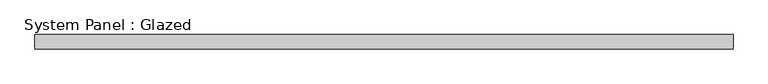
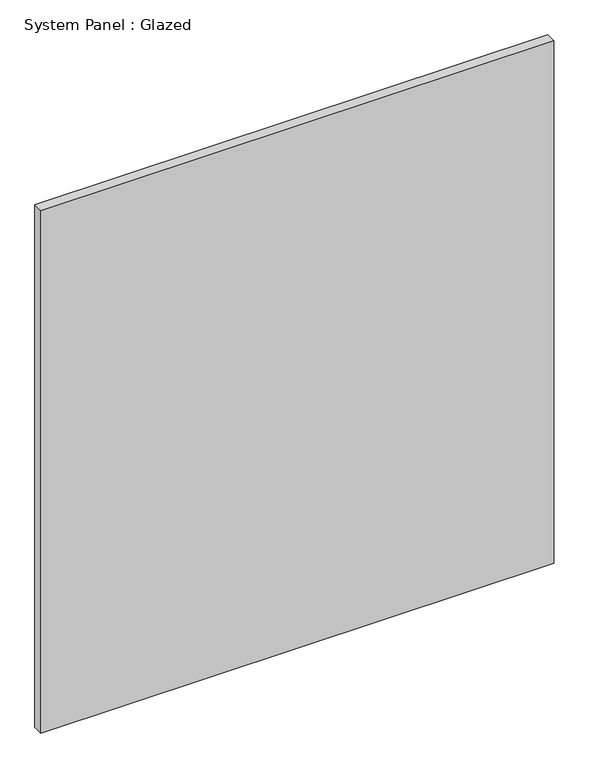
"""IFC4 building model written with IfcOpenShell, lengths in millimetres: plate geometry, System Panel : Glazed."""

from ifc_helpers import new_model, si_unit, origin, origin_with_axes, place, context, project, spatial, polyline, outline, extrude, source, transform, mapped, element, save


def system_panel_glazed_bb4db1d5(model_context):
    return source(origin(), model_context, "Body", "SweptSolid", [
        extrude(outline(polyline([(618.0666667, 24.5), (-618.0666667, 24.5), (-618.0666667, 49.5), (618.0666667, 49.5), (618.0666667, 24.5)])), origin_with_axes(), (0.0, 0.0, 1.0), 1330.8429687),
    ])


if __name__ == "__main__":
    model = new_model("IFC4")
    model_context = context("Model", 3, world=origin())
    ifc_project = project(units=[si_unit("LENGTHUNIT", "METRE", prefix="MILLI")], contexts=[model_context])
    site = spatial("IfcSite", under=ifc_project)
    building = spatial("IfcBuilding", under=site)
    placement = place(None, origin())
    system_panel_glazed_shape = system_panel_glazed_bb4db1d5(model_context)
    element("IfcPlate", 1, ObjectType="System Panel : Glazed", at=placement, inside=building, context=model_context, shape_type="MappedRepresentation", body=[
        mapped(system_panel_glazed_shape, transform((0.0, 0.0, 0.0), x_axis=(1.0, 0.0, 0.0), y_axis=(0.0, 1.0, 0.0), z_axis=(0.0, 0.0, 1.0))),
    ])
    save(model, "model.ifc")

# Revit data of these elements
# Type "System Panel : Glazed"
#   Keynote = "H11"
#   Construction Type Id = "GSP4R"
#   Analytic Construction = "1/8 in Pilkington single glazing"
#   Visual Light Transmittance = 0.9
#   Solar Heat Gain Coefficient = 0.86
#   Heat Transfer Coefficient (U) = 6.7069 W/(m²·K)
#   Define Thermal Properties by = 1
# Element 1 (IfcPlate, "System Panel : Glazed")
#   Materials on its faces: "Glass"
# Materials
#   "Glass": class "Glass", colour RGB 0 128 192, transparency 0.9, Description = "Soda Lime Glass", Cost = 0
